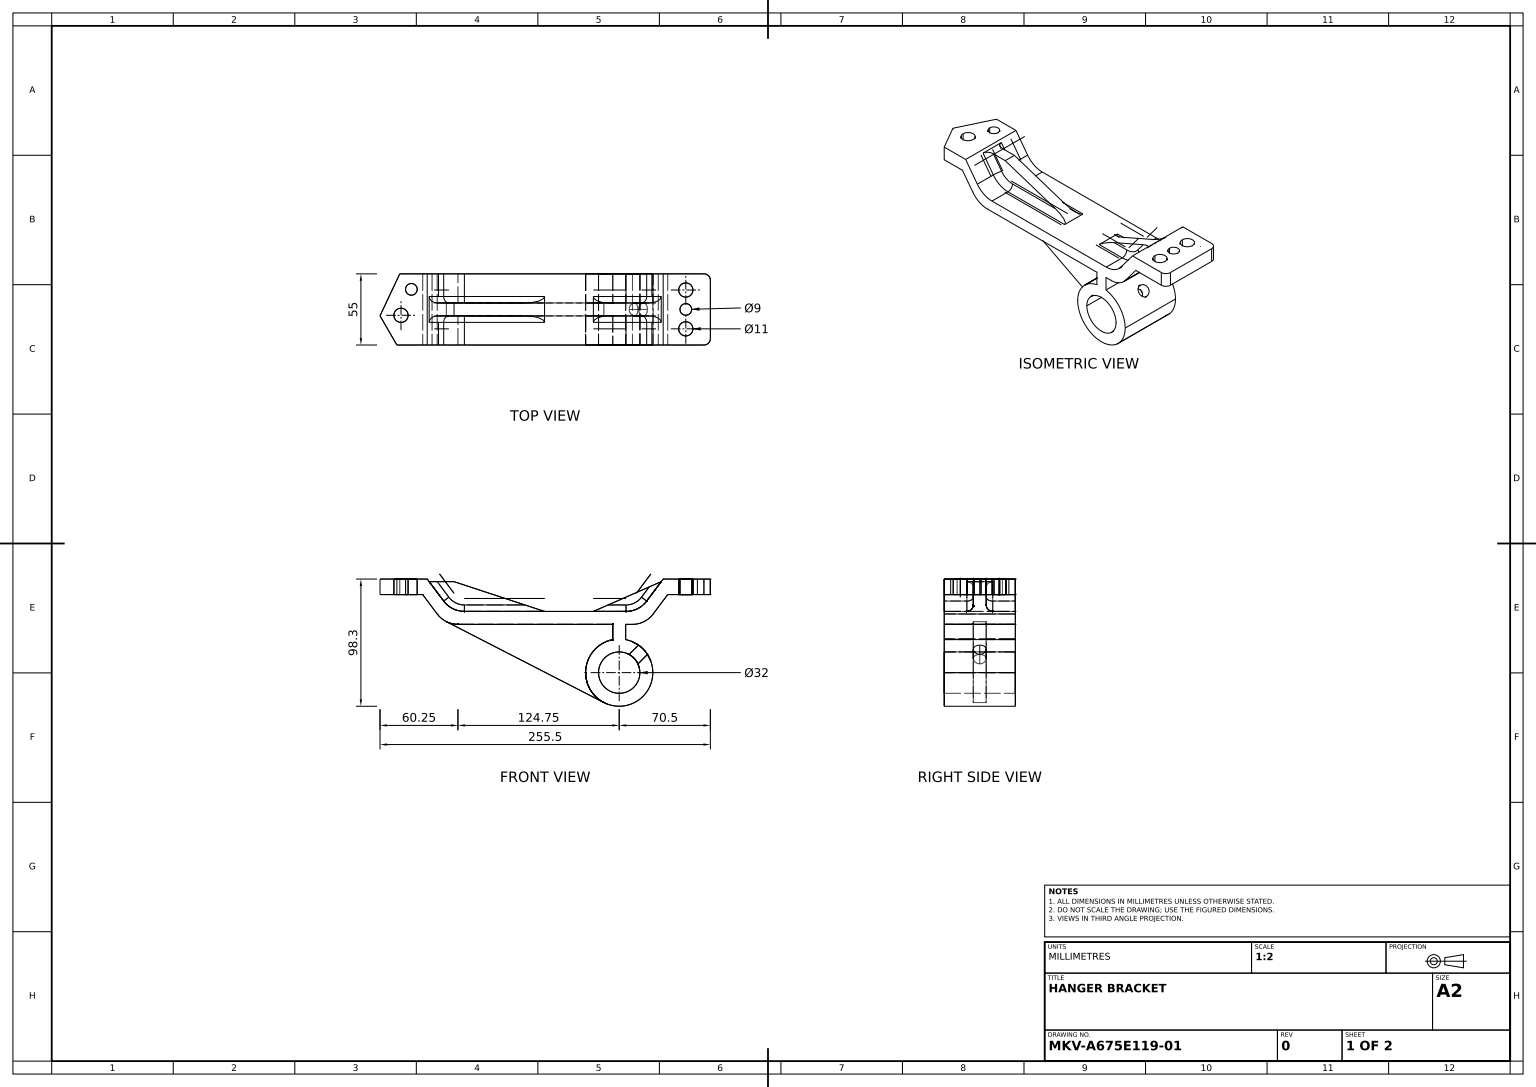
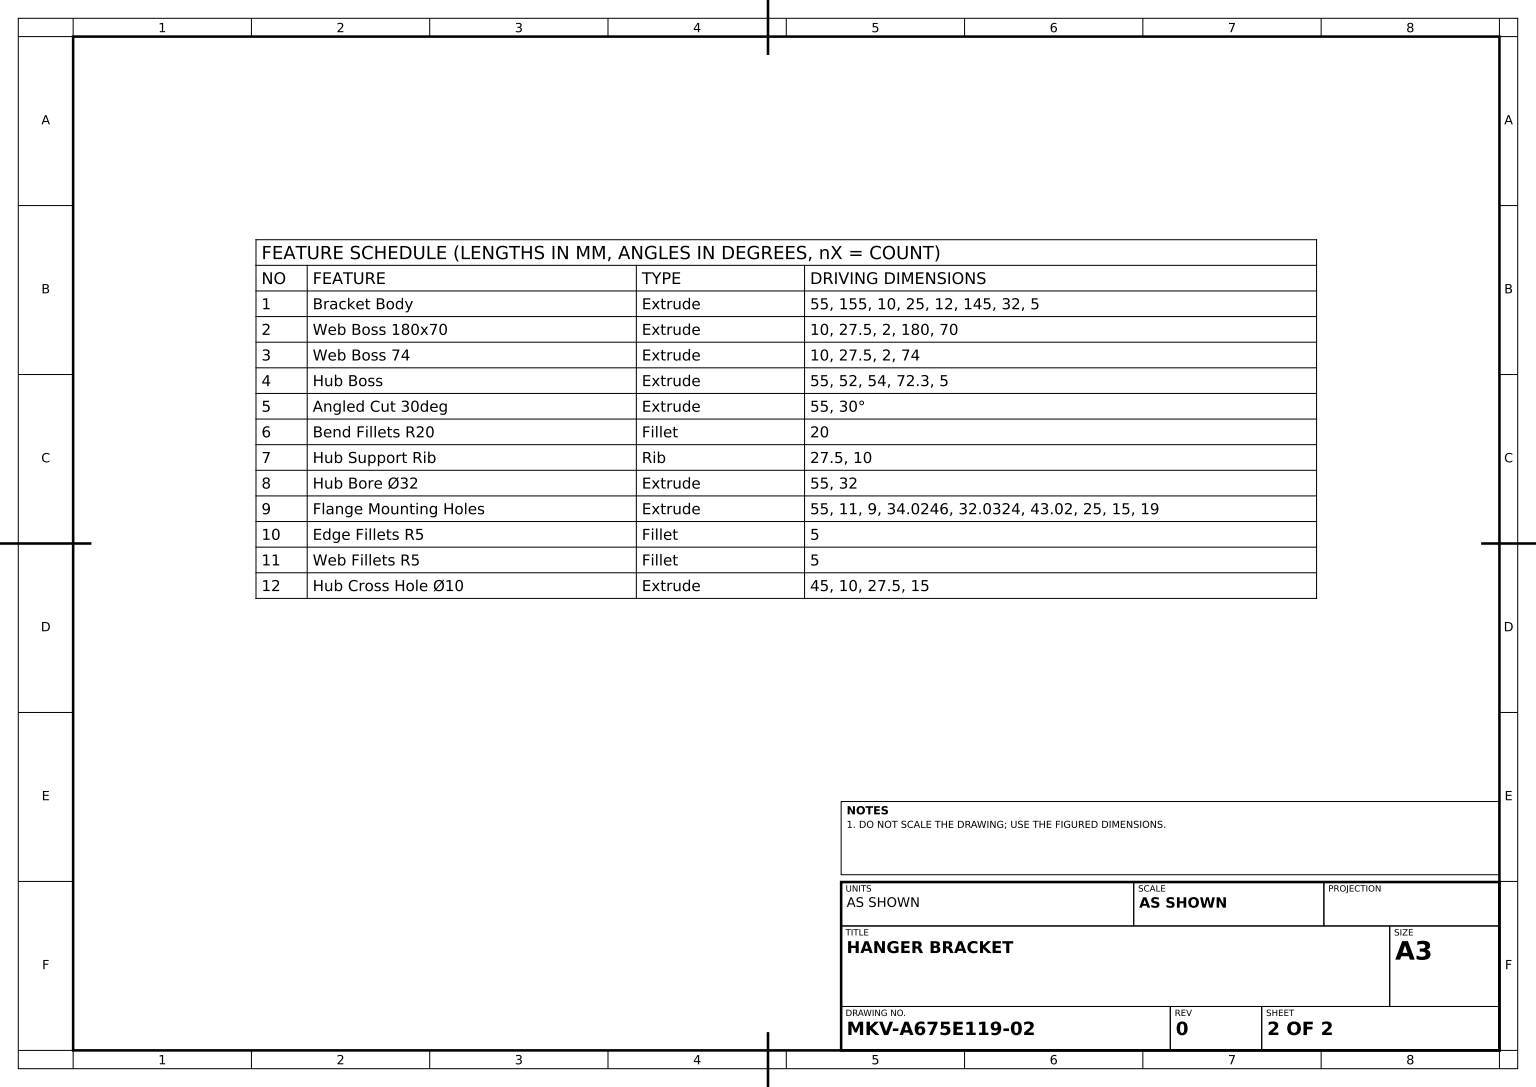
SolidWorks part; units mm, degrees
material "Plain Carbon Steel"
ref_plane "Front Plane" through (0, 0, 0) normal (0, 0, 1) x (1, 0, 0)
ref_plane "Top Plane" through (0, 0, 0) normal (0, 1, 0) x (1, 0, 0)
ref_plane "Right Plane" through (0, 0, 0) normal (1, 0, 0) x (0, 0, -1)
sketch "Bracket Profile Sketch" plane through (0, 0, 0) normal (0, 0, 1) x (1, 0, 0)
  line L0 (0, 0) -> (155, 0)
  line L1 (0, 0) -> (-17.25, 23)
  line L2 (-17.25, 23) -> (-50.25, 23)
  line L3 (-50.25, 23) -> (-50.25, 35)
  line L4 (-50.25, 35) -> (-13.75, 35)
  line L5 (-13.75, 35) -> (5, 10)
  line L6 (5, 10) -> (150, 10)
  line L7 (150, 10) -> (168.75, 35)
  line L8 (168.75, 35) -> (205.25, 35)
  line L9 (205.25, 35) -> (205.25, 23)
  line L10 (155, 0) -> (172.25, 23)
  line L11 (172.25, 23) -> (205.25, 23)
  point P3 (187, 35)
  point P13 (-32, 35)
  dimension "D1" = 155
  dimension "D2" = 10
  dimension "D3" = 25
  dimension "D4" = 12
  dimension "D5" = 25
  dimension "D6" = 12
  dimension "D7" = 145
  dimension "D8" = 32
  dimension "D9" = 32
  dimension "D10" = 10
  dimension "D11" = 5
extrude "Bracket Body" add sketch "Bracket Profile Sketch" against normal blind 55
sketch "Web Boss 180x70 Sketch" plane through (0, 0, 0) normal (0, 0, 1) x (1, 0, 0)
  line L0 (-12.25, 33) -> (7, 33)
  line L1 (5, 10) -> (-13.75, 35) construction
  line L2 (7, 33) -> (77, 10)
  line L3 (150, 10) -> (5, 10) construction
  line L4 (-13.75, 35) -> (-50.25, 35) construction
  line L5 (205.25, 35) -> (168.75, 35) construction
  line L6 (-12.25, 33) -> (5, 10)
  line L7 (5, 10) -> (77, 10)
  point P11 (187, 35)
  dimension "D1" = 2
  dimension "D2" = 180
  dimension "D3" = 70
extrude "Web Boss 180x70" add sketch "Web Boss 180x70 Sketch" along normal mid plane 10 from offset 27.5 offset against normal yes
sketch "Web Boss 74 Sketch" plane through (0, 0, 0) normal (0, 0, 1) x (1, 0, 0)
  line L0 (167.25, 33) -> (114.75, 10)
  line L1 (168.75, 35) -> (150, 10) construction
  line L2 (150, 10) -> (5, 10) construction
  line L3 (205.25, 35) -> (168.75, 35) construction
  line L4 (172.25, 23) -> (205.25, 23) construction
  line L5 (167.25, 33) -> (150, 10)
  line L6 (150, 10) -> (114.75, 10)
  point P10 (188.75, 23)
  dimension "D1" = 2
  dimension "D2" = 74
extrude "Web Boss 74" add sketch "Web Boss 74 Sketch" along normal mid plane 10 from offset 27.5 offset against normal yes
sketch "Hub Boss Sketch" plane through (0, 0, 0) normal (0, 0, 1) x (1, 0, 0)
  line L0 (172.25, 23) -> (205.25, 23) construction
  line L1 (205.25, 35) -> (168.75, 35) construction
  line L2 (134.75, -37.3) -> (134.75, 0) construction
  line L3 (0, 0) -> (155, 0) construction
  line L4 (139.75, -11.7853) -> (139.75, 0)
  line L5 (129.75, -11.7853) -> (129.75, 0)
  line L6 (129.75, 0) -> (139.75, 0)
  line L7 (129.75, -37.3) -> (129.75, 0) construction
  line L8 (139.75, -37.3) -> (139.75, 0) construction
  circle A0 centre (134.75, -37.3) radius 26
  point P4 (188.75, 23)
  line M3 (0, 0) -> (155, 0)
  dimension "D1" = 52
  dimension "D2" = 54
  dimension "D3" = 72.3
  dimension "D4" = 5
  dimension "D5" = 5
extrude "Hub Boss" add sketch "Hub Boss Sketch" against normal blind 55 contours A0 | A0 L4 L5 M3
sketch "Angled Cut Sketch" plane through (0, 35, 0) normal (0, 1, 0) x (1, 0, 0)
  line L0 (-50.25, 55) -> (-50.25, 0) construction
  line L1 (-50.25, 22.568) -> (-37.2204, 0)
  line L2 (-13.75, 0) -> (-50.25, 0) construction
  line L3 (-50.25, 22.568) -> (-50.25, 0) construction
  line L4 (-50.25, 22.568) -> (-34.992, 55)
  line L5 (-13.75, 55) -> (-50.25, 55) construction
  line L6 (-34.992, 55) -> (-13.75, 55)
  line L7 (-13.75, 55) -> (-13.75, 0)
  line L8 (-13.75, 0) -> (-37.2204, 0)
  line L9 (-13.75, 55) -> (-13.75, 0) construction
  line M7 (-50.25, 0) -> (-13.75, 0)
  line M9 (-13.75, 55) -> (-50.25, 55)
  line M10 (-50.25, 55) -> (-50.25, 0)
  dimension "D1" = 30
  dimension "D2" = 21.242
  dimension "D3" = 23.4704
extrude "Angled Cut 30deg" cut sketch "Angled Cut Sketch" against normal blind 55 contours L4 M10 M9 | L1 M10 M7
fillet "Bend Fillets R20" radius 20 6 edges at (155, 0, -27.5) (150, 10, -43.75) (150, 10, -11.25) (5, 10, -43.75) (0, 0, -27.5) (5, 10, -11.25)
ref_plane "Rib Plane" through (0, 0, -27.5) normal (0, 0, 1) x (1, 0, 0)
sketch "Support Rib Sketch" plane through (0, 0, -27.5) normal (0, 0, 1) x (1, 0, 0)
  line L0 (1.0557, 2.1115) -> (122.8753, -60.4299)
  arc A0 (-6, 8) -> (10, 0) centre (10, 20) ccw construction
  arc A1 (129.75, -11.7853) -> (139.75, -11.7853) centre (134.75, -37.3) ccw construction
rib "Hub Support Rib" sketch "Support Rib Sketch" sketch "Support Rib Sketch" thickness 10 extrusion direction parallel to sketch draft on no parameters "D1"=10
sketch "Hub Bore Sketch" plane through (0, 0, 0) normal (0, 0, 1) x (1, 0, 0)
  circle A0 centre (134.75, -37.3) radius 16
  dimension "D1" = 32
extrude "Hub Bore Ø32" cut sketch "Hub Bore Sketch" against normal blind 55
sketch "Flange Holes Sketch" plane through (0, 35, 0) normal (0, 1, 0) x (1, 0, 0)
  line L0 (-13.75, 55) -> (-34.992, 55) construction
  line L2 (205.25, 55) -> (205.25, 0) construction
  circle A0 centre (-34.0246, 22.9676) radius 5.5
  circle A1 centre (-26, 43.02) radius 4.5
  circle A2 centre (186.25, 42.5) radius 5.5
  circle A3 centre (186.25, 27.5) radius 4.5
  circle A4 centre (186.25, 12.5) radius 5.5
  point P17 (205.25, 27.5)
  dimension "D1" = 11
  dimension "D2" = 9
  dimension "D7" = 11
  dimension "D10" = 9
  dimension "D3" = 34.0246
  dimension "D4" = 32.0324
  dimension "D5" = 43.02
  dimension "D6" = 25
  dimension "D8" = 15
  dimension "D9" = 15
  dimension "D11" = 19
extrude "Flange Mounting Holes" cut sketch "Flange Holes Sketch" against normal blind 55
fillet "Edge Fillets R5" radius 5 2 edges at (205.25, 29, -55) (205.25, 29, 0)
fillet "Web Fillets R5" radius 5 12 edges at (161.625, 25.5, -22.5) (148.9443, 12.1115, -22.5) (161.625, 25.5, -32.5) (148.9443, 12.1115, -32.5) (46, 10, -32.5) (-6.625, 25.5, -32.5) (46, 10, -22.5) (6.0557, 12.1115, -22.5) (127.375, 10, -22.5) (127.375, 10, -32.5) (6.0557, 12.1115, -32.5) (-6.625, 25.5, -22.5)
sketch "Cross Hole Plane Line 45deg" plane through (0, 0, 0) normal (0, 0, 1) x (1, 0, 0)
  line L0 (134.75, -37.3) -> (163.5669, -8.4831) construction
  dimension "D1" = 45
ref_plane "Cross Hole Plane" through (163.5669, -8.4831, 0) normal (0.7071, 0.7071, 0) x (0.7071, -0.7071, 0)
sketch "Cross Hole Sketch" plane through (163.5669, -8.4831, 0) normal (0.7071, 0.7071, 0) x (0.7071, -0.7071, 0)
  line L0 (-26, 0) -> (26, 0) construction
  line L1 (-14.5061, 55) -> (-14.5061, 0) construction
  circle A0 centre (0.4939, 27.5) radius 5
  dimension "D1" = 27.5
  dimension "10" = 10
  dimension "D2" = 15
extrude "Hub Cross Hole Ø10" cut sketch "Cross Hole Sketch" against normal blind 45 contours A0
